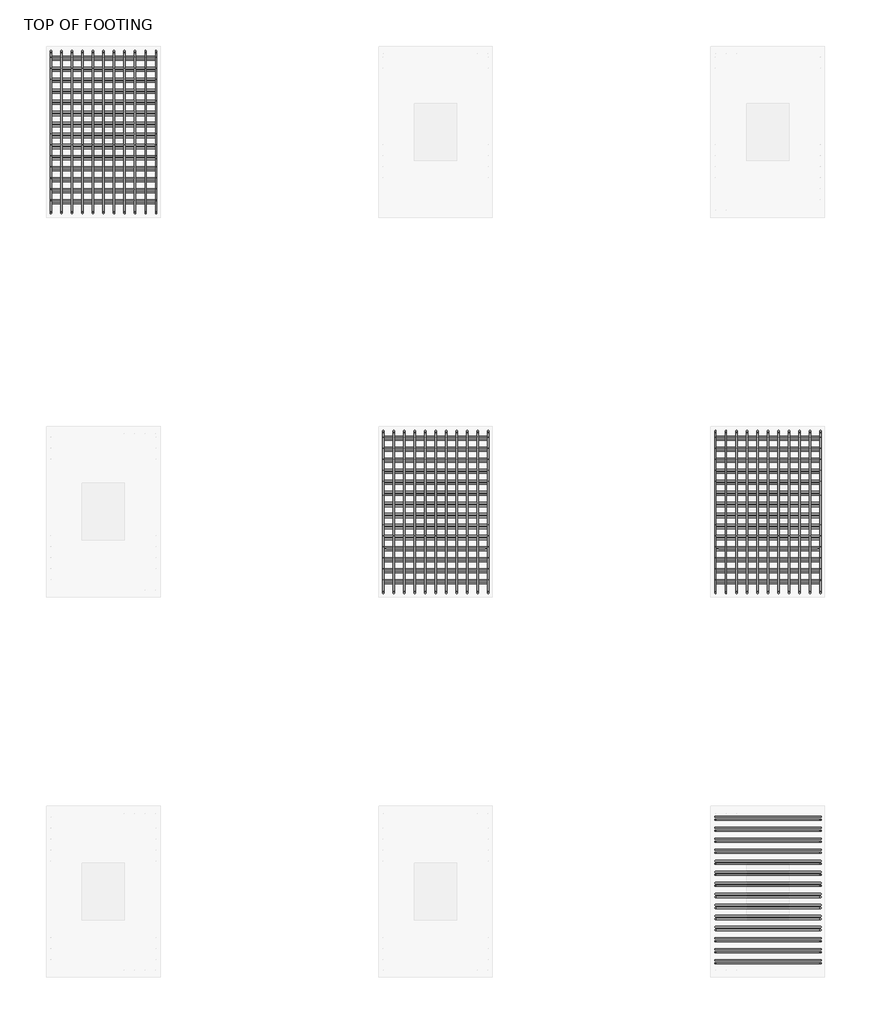
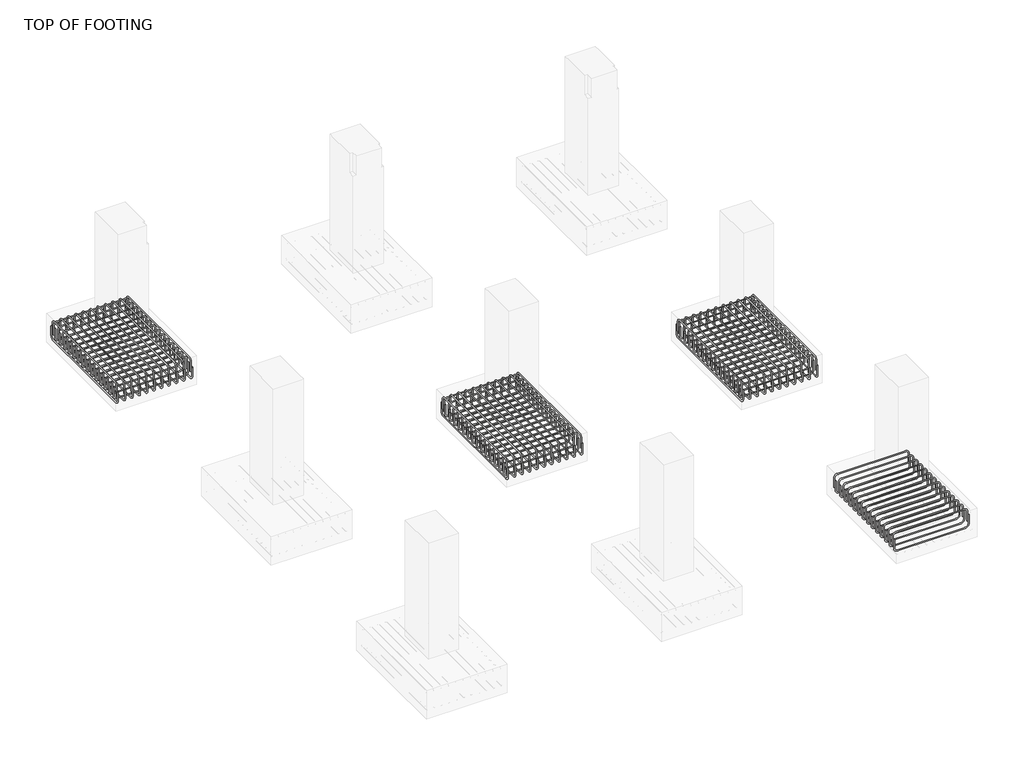
# One storey, part 4 of 11: 14 reinforcing bars.
"""IFC4 building model written with IfcOpenShell, lengths in millimetres."""

from ifc_helpers import new_model, si_unit, point, frame, origin, place, context, project, spatial, polyline, circle_curve, trimmed, segment, composite_curve, source, transform, mapped, element, save
from ifc_brep_helpers import swept_disk

model = new_model("IFC4")

# Units and contexts
model_context = context("Model", 3, world=origin())
ifc_project = project(units=[si_unit("LENGTHUNIT", "METRE", prefix="MILLI")], contexts=[model_context])

# Site, building, storey
site = spatial("IfcSite", under=ifc_project)
building = spatial("IfcBuilding", under=site)
storey = spatial("IfcBuildingStorey", under=building, Name="TOP OF FOOTING", Elevation=-1828.8)

# Reinforcing bars
placement = place(None, origin())
reinforcing_bar_shape = source(origin(), model_context, "Body", "SolidModel", [
    swept_disk(composite_curve([segment(polyline([(-8816.2384094, 10549.4712443, -2012.1658531), (-8816.2384094, 10549.4712443, -2159.4658531)]), True, "CONTINUOUS"), segment(trimmed(circle_curve(frame((-8816.2384094, 10595.8212443, -2159.4658531), z_axis=(1.0, 0.0, 0.0), x_axis=(0.0, -46.349999999998545, 0.0)), 46.35), [point((-8816.2384094, 10549.4712443, -2159.4658531))], [point((-8816.2384094, 10595.8212443, -2205.8158531))], True, "CARTESIAN"), True, "CONTINUOUS"), segment(polyline([(-8816.2384094, 10595.8212443, -2205.8158531), (-8816.2384094, 12210.4212443, -2205.8158531)]), True, "CONTINUOUS"), segment(trimmed(circle_curve(frame((-8816.2384094, 12210.4212443, -2159.4658531), z_axis=(1.0, 0.0, 0.0), x_axis=(0.0, 0.0, -46.34999999999991)), 46.35), [point((-8816.2384094, 12210.4212443, -2205.8158531))], [point((-8816.2384094, 12256.7712443, -2159.4658531))], True, "CARTESIAN"), True, "CONTINUOUS"), segment(polyline([(-8816.2384094, 12256.7712443, -2159.4658531), (-8816.2384094, 12256.7712443, -2012.1658531)]), True, "CONTINUOUS")], self_intersect=False), 6.35),
])
element("IfcReinforcingBar", 1, at=placement, inside=storey, context=model_context, shape_type="MappedRepresentation", body=[
    mapped(reinforcing_bar_shape, transform((0.0, 0.0, 0.0), x_axis=(1.0, 0.0, 0.0), y_axis=(0.0, 1.0, 0.0), z_axis=(0.0, 0.0, 1.0))),
    mapped(reinforcing_bar_shape, transform((-110.73, 0.0, 0.0), x_axis=(1.0, 0.0, 0.0), y_axis=(0.0, 1.0, 0.0), z_axis=(0.0, 0.0, 1.0))),
    mapped(reinforcing_bar_shape, transform((-221.46, 0.0, 0.0), x_axis=(1.0, 0.0, 0.0), y_axis=(0.0, 1.0, 0.0), z_axis=(0.0, 0.0, 1.0))),
    mapped(reinforcing_bar_shape, transform((-332.19, 0.0, 0.0), x_axis=(1.0, 0.0, 0.0), y_axis=(0.0, 1.0, 0.0), z_axis=(0.0, 0.0, 1.0))),
    mapped(reinforcing_bar_shape, transform((-442.92, 0.0, 0.0), x_axis=(1.0, 0.0, 0.0), y_axis=(0.0, 1.0, 0.0), z_axis=(0.0, 0.0, 1.0))),
    mapped(reinforcing_bar_shape, transform((-553.65, 0.0, 0.0), x_axis=(1.0, 0.0, 0.0), y_axis=(0.0, 1.0, 0.0), z_axis=(0.0, 0.0, 1.0))),
    mapped(reinforcing_bar_shape, transform((-664.38, 0.0, 0.0), x_axis=(1.0, 0.0, 0.0), y_axis=(0.0, 1.0, 0.0), z_axis=(0.0, 0.0, 1.0))),
    mapped(reinforcing_bar_shape, transform((-775.11, 0.0, 0.0), x_axis=(1.0, 0.0, 0.0), y_axis=(0.0, 1.0, 0.0), z_axis=(0.0, 0.0, 1.0))),
    mapped(reinforcing_bar_shape, transform((-885.84, 0.0, 0.0), x_axis=(1.0, 0.0, 0.0), y_axis=(0.0, 1.0, 0.0), z_axis=(0.0, 0.0, 1.0))),
    mapped(reinforcing_bar_shape, transform((-996.57, 0.0, 0.0), x_axis=(1.0, 0.0, 0.0), y_axis=(0.0, 1.0, 0.0), z_axis=(0.0, 0.0, 1.0))),
    mapped(reinforcing_bar_shape, transform((-1107.3, 0.0, 0.0), x_axis=(1.0, 0.0, 0.0), y_axis=(0.0, 1.0, 0.0), z_axis=(0.0, 0.0, 1.0))),
])
reinforcing_bar_2_shape = source(origin(), model_context, "Body", "SolidModel", [
    swept_disk(composite_curve([segment(polyline([(-9923.5384094, 10577.6603603, -2096.8914539), (-9923.5384094, 10577.6603603, -1949.5914539)]), True, "CONTINUOUS"), segment(trimmed(circle_curve(frame((-9923.5384094, 10624.0103603, -1949.5914539), z_axis=(-1.0, 0.0, 0.0), x_axis=(0.0, -46.350000000000364, 0.0)), 46.35), [point((-9923.5384094, 10577.6603603, -1949.5914539))], [point((-9923.5384094, 10624.0103603, -1903.2414539))], True, "CARTESIAN"), True, "CONTINUOUS"), segment(polyline([(-9923.5384094, 10624.0103603, -1903.2414539), (-9923.5384094, 12181.3238837, -1903.2414539)]), True, "CONTINUOUS"), segment(trimmed(circle_curve(frame((-9923.5384094, 12181.3238837, -1949.5914539), z_axis=(-1.0, 0.0, 0.0), x_axis=(0.0, 0.0, 46.350000000000136)), 46.35), [point((-9923.5384094, 12181.3238837, -1903.2414539))], [point((-9923.5384094, 12227.6738837, -1949.5914539))], True, "CARTESIAN"), True, "CONTINUOUS"), segment(polyline([(-9923.5384094, 12227.6738837, -1949.5914539), (-9923.5384094, 12227.6738837, -2096.8914539)]), True, "CONTINUOUS")], self_intersect=False), 6.35),
])
element("IfcReinforcingBar", 2, at=placement, inside=storey, context=model_context, shape_type="MappedRepresentation", body=[
    mapped(reinforcing_bar_2_shape, transform((0.0, 0.0, 0.0), x_axis=(1.0, 0.0, 0.0), y_axis=(0.0, 1.0, 0.0), z_axis=(0.0, 0.0, 1.0))),
    mapped(reinforcing_bar_2_shape, transform((110.73, 0.0, 0.0), x_axis=(1.0, 0.0, 0.0), y_axis=(0.0, 1.0, 0.0), z_axis=(0.0, 0.0, 1.0))),
    mapped(reinforcing_bar_2_shape, transform((221.46, 0.0, 0.0), x_axis=(1.0, 0.0, 0.0), y_axis=(0.0, 1.0, 0.0), z_axis=(0.0, 0.0, 1.0))),
    mapped(reinforcing_bar_2_shape, transform((332.19, 0.0, 0.0), x_axis=(1.0, 0.0, 0.0), y_axis=(0.0, 1.0, 0.0), z_axis=(0.0, 0.0, 1.0))),
    mapped(reinforcing_bar_2_shape, transform((442.92, 0.0, 0.0), x_axis=(1.0, 0.0, 0.0), y_axis=(0.0, 1.0, 0.0), z_axis=(0.0, 0.0, 1.0))),
    mapped(reinforcing_bar_2_shape, transform((553.65, 0.0, 0.0), x_axis=(1.0, 0.0, 0.0), y_axis=(0.0, 1.0, 0.0), z_axis=(0.0, 0.0, 1.0))),
    mapped(reinforcing_bar_2_shape, transform((664.38, 0.0, 0.0), x_axis=(1.0, 0.0, 0.0), y_axis=(0.0, 1.0, 0.0), z_axis=(0.0, 0.0, 1.0))),
    mapped(reinforcing_bar_2_shape, transform((775.11, 0.0, 0.0), x_axis=(1.0, 0.0, 0.0), y_axis=(0.0, 1.0, 0.0), z_axis=(0.0, 0.0, 1.0))),
    mapped(reinforcing_bar_2_shape, transform((885.84, 0.0, 0.0), x_axis=(1.0, 0.0, 0.0), y_axis=(0.0, 1.0, 0.0), z_axis=(0.0, 0.0, 1.0))),
    mapped(reinforcing_bar_2_shape, transform((996.57, 0.0, 0.0), x_axis=(1.0, 0.0, 0.0), y_axis=(0.0, 1.0, 0.0), z_axis=(0.0, 0.0, 1.0))),
    mapped(reinforcing_bar_2_shape, transform((1107.3, 0.0, 0.0), x_axis=(1.0, 0.0, 0.0), y_axis=(0.0, 1.0, 0.0), z_axis=(0.0, 0.0, 1.0))),
])
reinforcing_bar_3_shape = source(origin(), model_context, "Body", "SolidModel", [
    swept_disk(composite_curve([segment(polyline([(-9923.5384094, 10653.1930221, -1996.7664426), (-9923.5384094, 10653.1930221, -2144.0664426)]), True, "CONTINUOUS"), segment(trimmed(circle_curve(frame((-9877.1884094, 10653.1930221, -2144.0664426), z_axis=(0.0, -1.0, 0.0), x_axis=(-46.350000000000364, 0.0, 0.0)), 46.35), [point((-9923.5384094, 10653.1930221, -2144.0664426))], [point((-9877.1884094, 10653.1930221, -2190.4164426))], True, "CARTESIAN"), True, "CONTINUOUS"), segment(polyline([(-9877.1884094, 10653.1930221, -2190.4164426), (-8862.5884094, 10653.1930221, -2190.4164426)]), True, "CONTINUOUS"), segment(trimmed(circle_curve(frame((-8862.5884094, 10653.1930221, -2144.0664426), z_axis=(0.0, -1.0, 0.0), x_axis=(0.0, 0.0, -46.350000000000364)), 46.35), [point((-8862.5884094, 10653.1930221, -2190.4164426))], [point((-8816.2384094, 10653.1930221, -2144.0664426))], True, "CARTESIAN"), True, "CONTINUOUS"), segment(polyline([(-8816.2384094, 10653.1930221, -2144.0664426), (-8816.2384094, 10653.1930221, -1996.7664426)]), True, "CONTINUOUS")], self_intersect=False), 6.35),
])
element("IfcReinforcingBar", 3, at=placement, inside=storey, context=model_context, shape_type="MappedRepresentation", body=[
    mapped(reinforcing_bar_3_shape, transform((0.0, 0.0, 0.0), x_axis=(1.0, 0.0, 0.0), y_axis=(0.0, 1.0, 0.0), z_axis=(0.0, 0.0, 1.0))),
    mapped(reinforcing_bar_3_shape, transform((0.0, 116.2744005, 0.0), x_axis=(1.0, 0.0, 0.0), y_axis=(0.0, 1.0, 0.0), z_axis=(0.0, 0.0, 1.0))),
    mapped(reinforcing_bar_3_shape, transform((0.0, 232.5488009, 0.0), x_axis=(1.0, 0.0, 0.0), y_axis=(0.0, 1.0, 0.0), z_axis=(0.0, 0.0, 1.0))),
    mapped(reinforcing_bar_3_shape, transform((0.0, 348.8232014, 0.0), x_axis=(1.0, 0.0, 0.0), y_axis=(0.0, 1.0, 0.0), z_axis=(0.0, 0.0, 1.0))),
    mapped(reinforcing_bar_3_shape, transform((0.0, 465.0976018, 0.0), x_axis=(1.0, 0.0, 0.0), y_axis=(0.0, 1.0, 0.0), z_axis=(0.0, 0.0, 1.0))),
    mapped(reinforcing_bar_3_shape, transform((0.0, 581.3720023, 0.0), x_axis=(1.0, 0.0, 0.0), y_axis=(0.0, 1.0, 0.0), z_axis=(0.0, 0.0, 1.0))),
    mapped(reinforcing_bar_3_shape, transform((0.0, 697.6464027, 0.0), x_axis=(1.0, 0.0, 0.0), y_axis=(0.0, 1.0, 0.0), z_axis=(0.0, 0.0, 1.0))),
    mapped(reinforcing_bar_3_shape, transform((0.0, 813.9208032, 0.0), x_axis=(1.0, 0.0, 0.0), y_axis=(0.0, 1.0, 0.0), z_axis=(0.0, 0.0, 1.0))),
    mapped(reinforcing_bar_3_shape, transform((0.0, 930.1952036, 0.0), x_axis=(1.0, 0.0, 0.0), y_axis=(0.0, 1.0, 0.0), z_axis=(0.0, 0.0, 1.0))),
    mapped(reinforcing_bar_3_shape, transform((0.0, 1046.4696041, 0.0), x_axis=(1.0, 0.0, 0.0), y_axis=(0.0, 1.0, 0.0), z_axis=(0.0, 0.0, 1.0))),
    mapped(reinforcing_bar_3_shape, transform((0.0, 1162.7440045, 0.0), x_axis=(1.0, 0.0, 0.0), y_axis=(0.0, 1.0, 0.0), z_axis=(0.0, 0.0, 1.0))),
    mapped(reinforcing_bar_3_shape, transform((0.0, 1279.018405, 0.0), x_axis=(1.0, 0.0, 0.0), y_axis=(0.0, 1.0, 0.0), z_axis=(0.0, 0.0, 1.0))),
    mapped(reinforcing_bar_3_shape, transform((0.0, 1395.2928054, 0.0), x_axis=(1.0, 0.0, 0.0), y_axis=(0.0, 1.0, 0.0), z_axis=(0.0, 0.0, 1.0))),
    mapped(reinforcing_bar_3_shape, transform((0.0, 1511.5672059, 0.0), x_axis=(1.0, 0.0, 0.0), y_axis=(0.0, 1.0, 0.0), z_axis=(0.0, 0.0, 1.0))),
])
reinforcing_bar_4_shape = source(origin(), model_context, "Body", "SolidModel", [
    swept_disk(composite_curve([segment(polyline([(-9923.5384094, 12194.4257435, -2114.1958609), (-9923.5384094, 12194.4257435, -1966.8958609)]), True, "CONTINUOUS"), segment(trimmed(circle_curve(frame((-9877.1884094, 12194.4257435, -1966.8958609), z_axis=(0.0, 1.0, 0.0), x_axis=(-46.350000000000364, 0.0, 0.0)), 46.35), [point((-9923.5384094, 12194.4257435, -1966.8958609))], [point((-9877.1884094, 12194.4257435, -1920.5458609))], True, "CARTESIAN"), True, "CONTINUOUS"), segment(polyline([(-9877.1884094, 12194.4257435, -1920.5458609), (-8862.5884094, 12194.4257435, -1920.5458609)]), True, "CONTINUOUS"), segment(trimmed(circle_curve(frame((-8862.5884094, 12194.4257435, -1966.8958609), z_axis=(0.0, 1.0, 0.0), x_axis=(0.0, 0.0, 46.34999999999991)), 46.35), [point((-8862.5884094, 12194.4257435, -1920.5458609))], [point((-8816.2384094, 12194.4257435, -1966.8958609))], True, "CARTESIAN"), True, "CONTINUOUS"), segment(polyline([(-8816.2384094, 12194.4257435, -1966.8958609), (-8816.2384094, 12194.4257435, -2114.1958609)]), True, "CONTINUOUS")], self_intersect=False), 6.35),
])
element("IfcReinforcingBar", 4, at=placement, inside=storey, context=model_context, shape_type="MappedRepresentation", body=[
    mapped(reinforcing_bar_4_shape, transform((0.0, 0.0, 0.0), x_axis=(1.0, 0.0, 0.0), y_axis=(0.0, 1.0, 0.0), z_axis=(0.0, 0.0, 1.0))),
    mapped(reinforcing_bar_4_shape, transform((0.0, -116.1057918, 0.0), x_axis=(1.0, 0.0, 0.0), y_axis=(0.0, 1.0, 0.0), z_axis=(0.0, 0.0, 1.0))),
    mapped(reinforcing_bar_4_shape, transform((0.0, -232.2115836, 0.0), x_axis=(1.0, 0.0, 0.0), y_axis=(0.0, 1.0, 0.0), z_axis=(0.0, 0.0, 1.0))),
    mapped(reinforcing_bar_4_shape, transform((0.0, -348.3173754, 0.0), x_axis=(1.0, 0.0, 0.0), y_axis=(0.0, 1.0, 0.0), z_axis=(0.0, 0.0, 1.0))),
    mapped(reinforcing_bar_4_shape, transform((0.0, -464.4231672, 0.0), x_axis=(1.0, 0.0, 0.0), y_axis=(0.0, 1.0, 0.0), z_axis=(0.0, 0.0, 1.0))),
    mapped(reinforcing_bar_4_shape, transform((0.0, -580.528959, 0.0), x_axis=(1.0, 0.0, 0.0), y_axis=(0.0, 1.0, 0.0), z_axis=(0.0, 0.0, 1.0))),
    mapped(reinforcing_bar_4_shape, transform((0.0, -696.6347508, 0.0), x_axis=(1.0, 0.0, 0.0), y_axis=(0.0, 1.0, 0.0), z_axis=(0.0, 0.0, 1.0))),
    mapped(reinforcing_bar_4_shape, transform((0.0, -812.7405426, 0.0), x_axis=(1.0, 0.0, 0.0), y_axis=(0.0, 1.0, 0.0), z_axis=(0.0, 0.0, 1.0))),
    mapped(reinforcing_bar_4_shape, transform((0.0, -928.8463344, 0.0), x_axis=(1.0, 0.0, 0.0), y_axis=(0.0, 1.0, 0.0), z_axis=(0.0, 0.0, 1.0))),
    mapped(reinforcing_bar_4_shape, transform((0.0, -1044.9521262, 0.0), x_axis=(1.0, 0.0, 0.0), y_axis=(0.0, 1.0, 0.0), z_axis=(0.0, 0.0, 1.0))),
    mapped(reinforcing_bar_4_shape, transform((0.0, -1161.057918, 0.0), x_axis=(1.0, 0.0, 0.0), y_axis=(0.0, 1.0, 0.0), z_axis=(0.0, 0.0, 1.0))),
    mapped(reinforcing_bar_4_shape, transform((0.0, -1277.1637098, 0.0), x_axis=(1.0, 0.0, 0.0), y_axis=(0.0, 1.0, 0.0), z_axis=(0.0, 0.0, 1.0))),
    mapped(reinforcing_bar_4_shape, transform((0.0, -1393.2695016, 0.0), x_axis=(1.0, 0.0, 0.0), y_axis=(0.0, 1.0, 0.0), z_axis=(0.0, 0.0, 1.0))),
    mapped(reinforcing_bar_4_shape, transform((0.0, -1509.3752934, 0.0), x_axis=(1.0, 0.0, 0.0), y_axis=(0.0, 1.0, 0.0), z_axis=(0.0, 0.0, 1.0))),
])
reinforcing_bar_5_shape = source(origin(), model_context, "Body", "SolidModel", [
    swept_disk(composite_curve([segment(polyline([(-5316.2384094, 6549.4712443, -2012.1658531), (-5316.2384094, 6549.4712443, -2159.4658531)]), True, "CONTINUOUS"), segment(trimmed(circle_curve(frame((-5316.2384094, 6595.8212443, -2159.4658531), z_axis=(1.0, 0.0, 0.0), x_axis=(0.0, -46.350000000000364, 0.0)), 46.35), [point((-5316.2384094, 6549.4712443, -2159.4658531))], [point((-5316.2384094, 6595.8212443, -2205.8158531))], True, "CARTESIAN"), True, "CONTINUOUS"), segment(polyline([(-5316.2384094, 6595.8212443, -2205.8158531), (-5316.2384094, 8210.4212443, -2205.8158531)]), True, "CONTINUOUS"), segment(trimmed(circle_curve(frame((-5316.2384094, 8210.4212443, -2159.4658531), z_axis=(1.0, 0.0, 0.0), x_axis=(0.0, 0.0, -46.34999999999991)), 46.35), [point((-5316.2384094, 8210.4212443, -2205.8158531))], [point((-5316.2384094, 8256.7712443, -2159.4658531))], True, "CARTESIAN"), True, "CONTINUOUS"), segment(polyline([(-5316.2384094, 8256.7712443, -2159.4658531), (-5316.2384094, 8256.7712443, -2012.1658531)]), True, "CONTINUOUS")], self_intersect=False), 6.35),
])
element("IfcReinforcingBar", 5, at=placement, inside=storey, context=model_context, shape_type="MappedRepresentation", body=[
    mapped(reinforcing_bar_5_shape, transform((0.0, 0.0, 0.0), x_axis=(1.0, 0.0, 0.0), y_axis=(0.0, 1.0, 0.0), z_axis=(0.0, 0.0, 1.0))),
    mapped(reinforcing_bar_5_shape, transform((-110.73, 0.0, 0.0), x_axis=(1.0, 0.0, 0.0), y_axis=(0.0, 1.0, 0.0), z_axis=(0.0, 0.0, 1.0))),
    mapped(reinforcing_bar_5_shape, transform((-221.46, 0.0, 0.0), x_axis=(1.0, 0.0, 0.0), y_axis=(0.0, 1.0, 0.0), z_axis=(0.0, 0.0, 1.0))),
    mapped(reinforcing_bar_5_shape, transform((-332.19, 0.0, 0.0), x_axis=(1.0, 0.0, 0.0), y_axis=(0.0, 1.0, 0.0), z_axis=(0.0, 0.0, 1.0))),
    mapped(reinforcing_bar_5_shape, transform((-442.92, 0.0, 0.0), x_axis=(1.0, 0.0, 0.0), y_axis=(0.0, 1.0, 0.0), z_axis=(0.0, 0.0, 1.0))),
    mapped(reinforcing_bar_5_shape, transform((-553.65, 0.0, 0.0), x_axis=(1.0, 0.0, 0.0), y_axis=(0.0, 1.0, 0.0), z_axis=(0.0, 0.0, 1.0))),
    mapped(reinforcing_bar_5_shape, transform((-664.38, 0.0, 0.0), x_axis=(1.0, 0.0, 0.0), y_axis=(0.0, 1.0, 0.0), z_axis=(0.0, 0.0, 1.0))),
    mapped(reinforcing_bar_5_shape, transform((-775.11, 0.0, 0.0), x_axis=(1.0, 0.0, 0.0), y_axis=(0.0, 1.0, 0.0), z_axis=(0.0, 0.0, 1.0))),
    mapped(reinforcing_bar_5_shape, transform((-885.84, 0.0, 0.0), x_axis=(1.0, 0.0, 0.0), y_axis=(0.0, 1.0, 0.0), z_axis=(0.0, 0.0, 1.0))),
    mapped(reinforcing_bar_5_shape, transform((-996.57, 0.0, 0.0), x_axis=(1.0, 0.0, 0.0), y_axis=(0.0, 1.0, 0.0), z_axis=(0.0, 0.0, 1.0))),
    mapped(reinforcing_bar_5_shape, transform((-1107.3, 0.0, 0.0), x_axis=(1.0, 0.0, 0.0), y_axis=(0.0, 1.0, 0.0), z_axis=(0.0, 0.0, 1.0))),
])
reinforcing_bar_6_shape = source(origin(), model_context, "Body", "SolidModel", [
    swept_disk(composite_curve([segment(polyline([(-6423.5384094, 6577.6603603, -2096.8914539), (-6423.5384094, 6577.6603603, -1949.5914539)]), True, "CONTINUOUS"), segment(trimmed(circle_curve(frame((-6423.5384094, 6624.0103603, -1949.5914539), z_axis=(-1.0, 0.0, 0.0), x_axis=(0.0, -46.349999999999454, 0.0)), 46.35), [point((-6423.5384094, 6577.6603603, -1949.5914539))], [point((-6423.5384094, 6624.0103603, -1903.2414539))], True, "CARTESIAN"), True, "CONTINUOUS"), segment(polyline([(-6423.5384094, 6624.0103603, -1903.2414539), (-6423.5384094, 8181.3238837, -1903.2414539)]), True, "CONTINUOUS"), segment(trimmed(circle_curve(frame((-6423.5384094, 8181.3238837, -1949.5914539), z_axis=(-1.0, 0.0, 0.0), x_axis=(0.0, 0.0, 46.350000000000136)), 46.35), [point((-6423.5384094, 8181.3238837, -1903.2414539))], [point((-6423.5384094, 8227.6738837, -1949.5914539))], True, "CARTESIAN"), True, "CONTINUOUS"), segment(polyline([(-6423.5384094, 8227.6738837, -1949.5914539), (-6423.5384094, 8227.6738837, -2096.8914539)]), True, "CONTINUOUS")], self_intersect=False), 6.35),
])
element("IfcReinforcingBar", 6, at=placement, inside=storey, context=model_context, shape_type="MappedRepresentation", body=[
    mapped(reinforcing_bar_6_shape, transform((0.0, 0.0, 0.0), x_axis=(1.0, 0.0, 0.0), y_axis=(0.0, 1.0, 0.0), z_axis=(0.0, 0.0, 1.0))),
    mapped(reinforcing_bar_6_shape, transform((110.73, 0.0, 0.0), x_axis=(1.0, 0.0, 0.0), y_axis=(0.0, 1.0, 0.0), z_axis=(0.0, 0.0, 1.0))),
    mapped(reinforcing_bar_6_shape, transform((221.46, 0.0, 0.0), x_axis=(1.0, 0.0, 0.0), y_axis=(0.0, 1.0, 0.0), z_axis=(0.0, 0.0, 1.0))),
    mapped(reinforcing_bar_6_shape, transform((332.19, 0.0, 0.0), x_axis=(1.0, 0.0, 0.0), y_axis=(0.0, 1.0, 0.0), z_axis=(0.0, 0.0, 1.0))),
    mapped(reinforcing_bar_6_shape, transform((442.92, 0.0, 0.0), x_axis=(1.0, 0.0, 0.0), y_axis=(0.0, 1.0, 0.0), z_axis=(0.0, 0.0, 1.0))),
    mapped(reinforcing_bar_6_shape, transform((553.65, 0.0, 0.0), x_axis=(1.0, 0.0, 0.0), y_axis=(0.0, 1.0, 0.0), z_axis=(0.0, 0.0, 1.0))),
    mapped(reinforcing_bar_6_shape, transform((664.38, 0.0, 0.0), x_axis=(1.0, 0.0, 0.0), y_axis=(0.0, 1.0, 0.0), z_axis=(0.0, 0.0, 1.0))),
    mapped(reinforcing_bar_6_shape, transform((775.11, 0.0, 0.0), x_axis=(1.0, 0.0, 0.0), y_axis=(0.0, 1.0, 0.0), z_axis=(0.0, 0.0, 1.0))),
    mapped(reinforcing_bar_6_shape, transform((885.84, 0.0, 0.0), x_axis=(1.0, 0.0, 0.0), y_axis=(0.0, 1.0, 0.0), z_axis=(0.0, 0.0, 1.0))),
    mapped(reinforcing_bar_6_shape, transform((996.57, 0.0, 0.0), x_axis=(1.0, 0.0, 0.0), y_axis=(0.0, 1.0, 0.0), z_axis=(0.0, 0.0, 1.0))),
    mapped(reinforcing_bar_6_shape, transform((1107.3, 0.0, 0.0), x_axis=(1.0, 0.0, 0.0), y_axis=(0.0, 1.0, 0.0), z_axis=(0.0, 0.0, 1.0))),
])
reinforcing_bar_7_shape = source(origin(), model_context, "Body", "SolidModel", [
    swept_disk(composite_curve([segment(polyline([(-6423.5384094, 6653.1930221, -1996.7664426), (-6423.5384094, 6653.1930221, -2144.0664426)]), True, "CONTINUOUS"), segment(trimmed(circle_curve(frame((-6377.1884094, 6653.1930221, -2144.0664426), z_axis=(0.0, -1.0, 0.0), x_axis=(-46.350000000000364, 0.0, 0.0)), 46.35), [point((-6423.5384094, 6653.1930221, -2144.0664426))], [point((-6377.1884094, 6653.1930221, -2190.4164426))], True, "CARTESIAN"), True, "CONTINUOUS"), segment(polyline([(-6377.1884094, 6653.1930221, -2190.4164426), (-5362.5884094, 6653.1930221, -2190.4164426)]), True, "CONTINUOUS"), segment(trimmed(circle_curve(frame((-5362.5884094, 6653.1930221, -2144.0664426), z_axis=(0.0, -1.0, 0.0), x_axis=(0.0, 0.0, -46.350000000000364)), 46.35), [point((-5362.5884094, 6653.1930221, -2190.4164426))], [point((-5316.2384094, 6653.1930221, -2144.0664426))], True, "CARTESIAN"), True, "CONTINUOUS"), segment(polyline([(-5316.2384094, 6653.1930221, -2144.0664426), (-5316.2384094, 6653.1930221, -1996.7664426)]), True, "CONTINUOUS")], self_intersect=False), 6.35),
])
element("IfcReinforcingBar", 7, at=placement, inside=storey, context=model_context, shape_type="MappedRepresentation", body=[
    mapped(reinforcing_bar_7_shape, transform((0.0, 0.0, 0.0), x_axis=(1.0, 0.0, 0.0), y_axis=(0.0, 1.0, 0.0), z_axis=(0.0, 0.0, 1.0))),
    mapped(reinforcing_bar_7_shape, transform((0.0, 116.2744005, 0.0), x_axis=(1.0, 0.0, 0.0), y_axis=(0.0, 1.0, 0.0), z_axis=(0.0, 0.0, 1.0))),
    mapped(reinforcing_bar_7_shape, transform((0.0, 232.5488009, 0.0), x_axis=(1.0, 0.0, 0.0), y_axis=(0.0, 1.0, 0.0), z_axis=(0.0, 0.0, 1.0))),
    mapped(reinforcing_bar_7_shape, transform((0.0, 348.8232014, 0.0), x_axis=(1.0, 0.0, 0.0), y_axis=(0.0, 1.0, 0.0), z_axis=(0.0, 0.0, 1.0))),
    mapped(reinforcing_bar_7_shape, transform((0.0, 465.0976018, 0.0), x_axis=(1.0, 0.0, 0.0), y_axis=(0.0, 1.0, 0.0), z_axis=(0.0, 0.0, 1.0))),
    mapped(reinforcing_bar_7_shape, transform((0.0, 581.3720023, 0.0), x_axis=(1.0, 0.0, 0.0), y_axis=(0.0, 1.0, 0.0), z_axis=(0.0, 0.0, 1.0))),
    mapped(reinforcing_bar_7_shape, transform((0.0, 697.6464027, 0.0), x_axis=(1.0, 0.0, 0.0), y_axis=(0.0, 1.0, 0.0), z_axis=(0.0, 0.0, 1.0))),
    mapped(reinforcing_bar_7_shape, transform((0.0, 813.9208032, 0.0), x_axis=(1.0, 0.0, 0.0), y_axis=(0.0, 1.0, 0.0), z_axis=(0.0, 0.0, 1.0))),
    mapped(reinforcing_bar_7_shape, transform((0.0, 930.1952036, 0.0), x_axis=(1.0, 0.0, 0.0), y_axis=(0.0, 1.0, 0.0), z_axis=(0.0, 0.0, 1.0))),
    mapped(reinforcing_bar_7_shape, transform((0.0, 1046.4696041, 0.0), x_axis=(1.0, 0.0, 0.0), y_axis=(0.0, 1.0, 0.0), z_axis=(0.0, 0.0, 1.0))),
    mapped(reinforcing_bar_7_shape, transform((0.0, 1162.7440045, 0.0), x_axis=(1.0, 0.0, 0.0), y_axis=(0.0, 1.0, 0.0), z_axis=(0.0, 0.0, 1.0))),
    mapped(reinforcing_bar_7_shape, transform((0.0, 1279.018405, 0.0), x_axis=(1.0, 0.0, 0.0), y_axis=(0.0, 1.0, 0.0), z_axis=(0.0, 0.0, 1.0))),
    mapped(reinforcing_bar_7_shape, transform((0.0, 1395.2928054, 0.0), x_axis=(1.0, 0.0, 0.0), y_axis=(0.0, 1.0, 0.0), z_axis=(0.0, 0.0, 1.0))),
    mapped(reinforcing_bar_7_shape, transform((0.0, 1511.5672059, 0.0), x_axis=(1.0, 0.0, 0.0), y_axis=(0.0, 1.0, 0.0), z_axis=(0.0, 0.0, 1.0))),
])
reinforcing_bar_8_shape = source(origin(), model_context, "Body", "SolidModel", [
    swept_disk(composite_curve([segment(polyline([(-6423.5384094, 8194.4257435, -2114.1958609), (-6423.5384094, 8194.4257435, -1966.8958609)]), True, "CONTINUOUS"), segment(trimmed(circle_curve(frame((-6377.1884094, 8194.4257435, -1966.8958609), z_axis=(0.0, 1.0, 0.0), x_axis=(-46.350000000000364, 0.0, 0.0)), 46.35), [point((-6423.5384094, 8194.4257435, -1966.8958609))], [point((-6377.1884094, 8194.4257435, -1920.5458609))], True, "CARTESIAN"), True, "CONTINUOUS"), segment(polyline([(-6377.1884094, 8194.4257435, -1920.5458609), (-5362.5884094, 8194.4257435, -1920.5458609)]), True, "CONTINUOUS"), segment(trimmed(circle_curve(frame((-5362.5884094, 8194.4257435, -1966.8958609), z_axis=(0.0, 1.0, 0.0), x_axis=(0.0, 0.0, 46.34999999999991)), 46.35), [point((-5362.5884094, 8194.4257435, -1920.5458609))], [point((-5316.2384094, 8194.4257435, -1966.8958609))], True, "CARTESIAN"), True, "CONTINUOUS"), segment(polyline([(-5316.2384094, 8194.4257435, -1966.8958609), (-5316.2384094, 8194.4257435, -2114.1958609)]), True, "CONTINUOUS")], self_intersect=False), 6.35),
])
element("IfcReinforcingBar", 8, at=placement, inside=storey, context=model_context, shape_type="MappedRepresentation", body=[
    mapped(reinforcing_bar_8_shape, transform((0.0, 0.0, 0.0), x_axis=(1.0, 0.0, 0.0), y_axis=(0.0, 1.0, 0.0), z_axis=(0.0, 0.0, 1.0))),
    mapped(reinforcing_bar_8_shape, transform((0.0, -116.1057918, 0.0), x_axis=(1.0, 0.0, 0.0), y_axis=(0.0, 1.0, 0.0), z_axis=(0.0, 0.0, 1.0))),
    mapped(reinforcing_bar_8_shape, transform((0.0, -232.2115836, 0.0), x_axis=(1.0, 0.0, 0.0), y_axis=(0.0, 1.0, 0.0), z_axis=(0.0, 0.0, 1.0))),
    mapped(reinforcing_bar_8_shape, transform((0.0, -348.3173754, 0.0), x_axis=(1.0, 0.0, 0.0), y_axis=(0.0, 1.0, 0.0), z_axis=(0.0, 0.0, 1.0))),
    mapped(reinforcing_bar_8_shape, transform((0.0, -464.4231672, 0.0), x_axis=(1.0, 0.0, 0.0), y_axis=(0.0, 1.0, 0.0), z_axis=(0.0, 0.0, 1.0))),
    mapped(reinforcing_bar_8_shape, transform((0.0, -580.528959, 0.0), x_axis=(1.0, 0.0, 0.0), y_axis=(0.0, 1.0, 0.0), z_axis=(0.0, 0.0, 1.0))),
    mapped(reinforcing_bar_8_shape, transform((0.0, -696.6347508, 0.0), x_axis=(1.0, 0.0, 0.0), y_axis=(0.0, 1.0, 0.0), z_axis=(0.0, 0.0, 1.0))),
    mapped(reinforcing_bar_8_shape, transform((0.0, -812.7405426, 0.0), x_axis=(1.0, 0.0, 0.0), y_axis=(0.0, 1.0, 0.0), z_axis=(0.0, 0.0, 1.0))),
    mapped(reinforcing_bar_8_shape, transform((0.0, -928.8463344, 0.0), x_axis=(1.0, 0.0, 0.0), y_axis=(0.0, 1.0, 0.0), z_axis=(0.0, 0.0, 1.0))),
    mapped(reinforcing_bar_8_shape, transform((0.0, -1044.9521262, 0.0), x_axis=(1.0, 0.0, 0.0), y_axis=(0.0, 1.0, 0.0), z_axis=(0.0, 0.0, 1.0))),
    mapped(reinforcing_bar_8_shape, transform((0.0, -1161.057918, 0.0), x_axis=(1.0, 0.0, 0.0), y_axis=(0.0, 1.0, 0.0), z_axis=(0.0, 0.0, 1.0))),
    mapped(reinforcing_bar_8_shape, transform((0.0, -1277.1637098, 0.0), x_axis=(1.0, 0.0, 0.0), y_axis=(0.0, 1.0, 0.0), z_axis=(0.0, 0.0, 1.0))),
    mapped(reinforcing_bar_8_shape, transform((0.0, -1393.2695016, 0.0), x_axis=(1.0, 0.0, 0.0), y_axis=(0.0, 1.0, 0.0), z_axis=(0.0, 0.0, 1.0))),
    mapped(reinforcing_bar_8_shape, transform((0.0, -1509.3752934, 0.0), x_axis=(1.0, 0.0, 0.0), y_axis=(0.0, 1.0, 0.0), z_axis=(0.0, 0.0, 1.0))),
])
reinforcing_bar_9_shape = source(origin(), model_context, "Body", "SolidModel", [
    swept_disk(composite_curve([segment(polyline([(-1816.2384094, 6549.4712443, -2012.1658531), (-1816.2384094, 6549.4712443, -2159.4658531)]), True, "CONTINUOUS"), segment(trimmed(circle_curve(frame((-1816.2384094, 6595.8212443, -2159.4658531), z_axis=(1.0, 0.0, 0.0), x_axis=(0.0, -46.350000000000364, 0.0)), 46.35), [point((-1816.2384094, 6549.4712443, -2159.4658531))], [point((-1816.2384094, 6595.8212443, -2205.8158531))], True, "CARTESIAN"), True, "CONTINUOUS"), segment(polyline([(-1816.2384094, 6595.8212443, -2205.8158531), (-1816.2384094, 8210.4212443, -2205.8158531)]), True, "CONTINUOUS"), segment(trimmed(circle_curve(frame((-1816.2384094, 8210.4212443, -2159.4658531), z_axis=(1.0, 0.0, 0.0), x_axis=(0.0, 0.0, -46.34999999999991)), 46.35), [point((-1816.2384094, 8210.4212443, -2205.8158531))], [point((-1816.2384094, 8256.7712443, -2159.4658531))], True, "CARTESIAN"), True, "CONTINUOUS"), segment(polyline([(-1816.2384094, 8256.7712443, -2159.4658531), (-1816.2384094, 8256.7712443, -2012.1658531)]), True, "CONTINUOUS")], self_intersect=False), 6.35),
])
element("IfcReinforcingBar", 9, at=placement, inside=storey, context=model_context, shape_type="MappedRepresentation", body=[
    mapped(reinforcing_bar_9_shape, transform((0.0, 0.0, 0.0), x_axis=(1.0, 0.0, 0.0), y_axis=(0.0, 1.0, 0.0), z_axis=(0.0, 0.0, 1.0))),
    mapped(reinforcing_bar_9_shape, transform((-110.73, 0.0, 0.0), x_axis=(1.0, 0.0, 0.0), y_axis=(0.0, 1.0, 0.0), z_axis=(0.0, 0.0, 1.0))),
    mapped(reinforcing_bar_9_shape, transform((-221.46, 0.0, 0.0), x_axis=(1.0, 0.0, 0.0), y_axis=(0.0, 1.0, 0.0), z_axis=(0.0, 0.0, 1.0))),
    mapped(reinforcing_bar_9_shape, transform((-332.19, 0.0, 0.0), x_axis=(1.0, 0.0, 0.0), y_axis=(0.0, 1.0, 0.0), z_axis=(0.0, 0.0, 1.0))),
    mapped(reinforcing_bar_9_shape, transform((-442.92, 0.0, 0.0), x_axis=(1.0, 0.0, 0.0), y_axis=(0.0, 1.0, 0.0), z_axis=(0.0, 0.0, 1.0))),
    mapped(reinforcing_bar_9_shape, transform((-553.65, 0.0, 0.0), x_axis=(1.0, 0.0, 0.0), y_axis=(0.0, 1.0, 0.0), z_axis=(0.0, 0.0, 1.0))),
    mapped(reinforcing_bar_9_shape, transform((-664.38, 0.0, 0.0), x_axis=(1.0, 0.0, 0.0), y_axis=(0.0, 1.0, 0.0), z_axis=(0.0, 0.0, 1.0))),
    mapped(reinforcing_bar_9_shape, transform((-775.11, 0.0, 0.0), x_axis=(1.0, 0.0, 0.0), y_axis=(0.0, 1.0, 0.0), z_axis=(0.0, 0.0, 1.0))),
    mapped(reinforcing_bar_9_shape, transform((-885.84, 0.0, 0.0), x_axis=(1.0, 0.0, 0.0), y_axis=(0.0, 1.0, 0.0), z_axis=(0.0, 0.0, 1.0))),
    mapped(reinforcing_bar_9_shape, transform((-996.57, 0.0, 0.0), x_axis=(1.0, 0.0, 0.0), y_axis=(0.0, 1.0, 0.0), z_axis=(0.0, 0.0, 1.0))),
    mapped(reinforcing_bar_9_shape, transform((-1107.3, 0.0, 0.0), x_axis=(1.0, 0.0, 0.0), y_axis=(0.0, 1.0, 0.0), z_axis=(0.0, 0.0, 1.0))),
])
reinforcing_bar_10_shape = source(origin(), model_context, "Body", "SolidModel", [
    swept_disk(composite_curve([segment(polyline([(-2923.5384094, 6577.6603603, -2096.8914539), (-2923.5384094, 6577.6603603, -1949.5914539)]), True, "CONTINUOUS"), segment(trimmed(circle_curve(frame((-2923.5384094, 6624.0103603, -1949.5914539), z_axis=(-1.0, 0.0, 0.0), x_axis=(0.0, -46.349999999999454, 0.0)), 46.35), [point((-2923.5384094, 6577.6603603, -1949.5914539))], [point((-2923.5384094, 6624.0103603, -1903.2414539))], True, "CARTESIAN"), True, "CONTINUOUS"), segment(polyline([(-2923.5384094, 6624.0103603, -1903.2414539), (-2923.5384094, 8181.3238837, -1903.2414539)]), True, "CONTINUOUS"), segment(trimmed(circle_curve(frame((-2923.5384094, 8181.3238837, -1949.5914539), z_axis=(-1.0, 0.0, 0.0), x_axis=(0.0, 0.0, 46.350000000000136)), 46.35), [point((-2923.5384094, 8181.3238837, -1903.2414539))], [point((-2923.5384094, 8227.6738837, -1949.5914539))], True, "CARTESIAN"), True, "CONTINUOUS"), segment(polyline([(-2923.5384094, 8227.6738837, -1949.5914539), (-2923.5384094, 8227.6738837, -2096.8914539)]), True, "CONTINUOUS")], self_intersect=False), 6.35),
])
element("IfcReinforcingBar", 10, at=placement, inside=storey, context=model_context, shape_type="MappedRepresentation", body=[
    mapped(reinforcing_bar_10_shape, transform((0.0, 0.0, 0.0), x_axis=(1.0, 0.0, 0.0), y_axis=(0.0, 1.0, 0.0), z_axis=(0.0, 0.0, 1.0))),
    mapped(reinforcing_bar_10_shape, transform((110.73, 0.0, 0.0), x_axis=(1.0, 0.0, 0.0), y_axis=(0.0, 1.0, 0.0), z_axis=(0.0, 0.0, 1.0))),
    mapped(reinforcing_bar_10_shape, transform((221.46, 0.0, 0.0), x_axis=(1.0, 0.0, 0.0), y_axis=(0.0, 1.0, 0.0), z_axis=(0.0, 0.0, 1.0))),
    mapped(reinforcing_bar_10_shape, transform((332.19, 0.0, 0.0), x_axis=(1.0, 0.0, 0.0), y_axis=(0.0, 1.0, 0.0), z_axis=(0.0, 0.0, 1.0))),
    mapped(reinforcing_bar_10_shape, transform((442.92, 0.0, 0.0), x_axis=(1.0, 0.0, 0.0), y_axis=(0.0, 1.0, 0.0), z_axis=(0.0, 0.0, 1.0))),
    mapped(reinforcing_bar_10_shape, transform((553.65, 0.0, 0.0), x_axis=(1.0, 0.0, 0.0), y_axis=(0.0, 1.0, 0.0), z_axis=(0.0, 0.0, 1.0))),
    mapped(reinforcing_bar_10_shape, transform((664.38, 0.0, 0.0), x_axis=(1.0, 0.0, 0.0), y_axis=(0.0, 1.0, 0.0), z_axis=(0.0, 0.0, 1.0))),
    mapped(reinforcing_bar_10_shape, transform((775.11, 0.0, 0.0), x_axis=(1.0, 0.0, 0.0), y_axis=(0.0, 1.0, 0.0), z_axis=(0.0, 0.0, 1.0))),
    mapped(reinforcing_bar_10_shape, transform((885.84, 0.0, 0.0), x_axis=(1.0, 0.0, 0.0), y_axis=(0.0, 1.0, 0.0), z_axis=(0.0, 0.0, 1.0))),
    mapped(reinforcing_bar_10_shape, transform((996.57, 0.0, 0.0), x_axis=(1.0, 0.0, 0.0), y_axis=(0.0, 1.0, 0.0), z_axis=(0.0, 0.0, 1.0))),
    mapped(reinforcing_bar_10_shape, transform((1107.3, 0.0, 0.0), x_axis=(1.0, 0.0, 0.0), y_axis=(0.0, 1.0, 0.0), z_axis=(0.0, 0.0, 1.0))),
])
reinforcing_bar_11_shape = source(origin(), model_context, "Body", "SolidModel", [
    swept_disk(composite_curve([segment(polyline([(-2923.5384094, 6653.1930221, -1996.7664426), (-2923.5384094, 6653.1930221, -2144.0664426)]), True, "CONTINUOUS"), segment(trimmed(circle_curve(frame((-2877.1884094, 6653.1930221, -2144.0664426), z_axis=(0.0, -1.0, 0.0), x_axis=(-46.34999999999991, 0.0, 0.0)), 46.35), [point((-2923.5384094, 6653.1930221, -2144.0664426))], [point((-2877.1884094, 6653.1930221, -2190.4164426))], True, "CARTESIAN"), True, "CONTINUOUS"), segment(polyline([(-2877.1884094, 6653.1930221, -2190.4164426), (-1862.5884094, 6653.1930221, -2190.4164426)]), True, "CONTINUOUS"), segment(trimmed(circle_curve(frame((-1862.5884094, 6653.1930221, -2144.0664426), z_axis=(0.0, -1.0, 0.0), x_axis=(0.0, 0.0, -46.350000000000364)), 46.35), [point((-1862.5884094, 6653.1930221, -2190.4164426))], [point((-1816.2384094, 6653.1930221, -2144.0664426))], True, "CARTESIAN"), True, "CONTINUOUS"), segment(polyline([(-1816.2384094, 6653.1930221, -2144.0664426), (-1816.2384094, 6653.1930221, -1996.7664426)]), True, "CONTINUOUS")], self_intersect=False), 6.35),
])
element("IfcReinforcingBar", 11, at=placement, inside=storey, context=model_context, shape_type="MappedRepresentation", body=[
    mapped(reinforcing_bar_11_shape, transform((0.0, 0.0, 0.0), x_axis=(1.0, 0.0, 0.0), y_axis=(0.0, 1.0, 0.0), z_axis=(0.0, 0.0, 1.0))),
    mapped(reinforcing_bar_11_shape, transform((0.0, 116.2744005, 0.0), x_axis=(1.0, 0.0, 0.0), y_axis=(0.0, 1.0, 0.0), z_axis=(0.0, 0.0, 1.0))),
    mapped(reinforcing_bar_11_shape, transform((0.0, 232.5488009, 0.0), x_axis=(1.0, 0.0, 0.0), y_axis=(0.0, 1.0, 0.0), z_axis=(0.0, 0.0, 1.0))),
    mapped(reinforcing_bar_11_shape, transform((0.0, 348.8232014, 0.0), x_axis=(1.0, 0.0, 0.0), y_axis=(0.0, 1.0, 0.0), z_axis=(0.0, 0.0, 1.0))),
    mapped(reinforcing_bar_11_shape, transform((0.0, 465.0976018, 0.0), x_axis=(1.0, 0.0, 0.0), y_axis=(0.0, 1.0, 0.0), z_axis=(0.0, 0.0, 1.0))),
    mapped(reinforcing_bar_11_shape, transform((0.0, 581.3720023, 0.0), x_axis=(1.0, 0.0, 0.0), y_axis=(0.0, 1.0, 0.0), z_axis=(0.0, 0.0, 1.0))),
    mapped(reinforcing_bar_11_shape, transform((0.0, 697.6464027, 0.0), x_axis=(1.0, 0.0, 0.0), y_axis=(0.0, 1.0, 0.0), z_axis=(0.0, 0.0, 1.0))),
    mapped(reinforcing_bar_11_shape, transform((0.0, 813.9208032, 0.0), x_axis=(1.0, 0.0, 0.0), y_axis=(0.0, 1.0, 0.0), z_axis=(0.0, 0.0, 1.0))),
    mapped(reinforcing_bar_11_shape, transform((0.0, 930.1952036, 0.0), x_axis=(1.0, 0.0, 0.0), y_axis=(0.0, 1.0, 0.0), z_axis=(0.0, 0.0, 1.0))),
    mapped(reinforcing_bar_11_shape, transform((0.0, 1046.4696041, 0.0), x_axis=(1.0, 0.0, 0.0), y_axis=(0.0, 1.0, 0.0), z_axis=(0.0, 0.0, 1.0))),
    mapped(reinforcing_bar_11_shape, transform((0.0, 1162.7440045, 0.0), x_axis=(1.0, 0.0, 0.0), y_axis=(0.0, 1.0, 0.0), z_axis=(0.0, 0.0, 1.0))),
    mapped(reinforcing_bar_11_shape, transform((0.0, 1279.018405, 0.0), x_axis=(1.0, 0.0, 0.0), y_axis=(0.0, 1.0, 0.0), z_axis=(0.0, 0.0, 1.0))),
    mapped(reinforcing_bar_11_shape, transform((0.0, 1395.2928054, 0.0), x_axis=(1.0, 0.0, 0.0), y_axis=(0.0, 1.0, 0.0), z_axis=(0.0, 0.0, 1.0))),
    mapped(reinforcing_bar_11_shape, transform((0.0, 1511.5672059, 0.0), x_axis=(1.0, 0.0, 0.0), y_axis=(0.0, 1.0, 0.0), z_axis=(0.0, 0.0, 1.0))),
])
reinforcing_bar_12_shape = source(origin(), model_context, "Body", "SolidModel", [
    swept_disk(composite_curve([segment(polyline([(-2923.5384094, 8194.4257435, -2114.1958609), (-2923.5384094, 8194.4257435, -1966.8958609)]), True, "CONTINUOUS"), segment(trimmed(circle_curve(frame((-2877.1884094, 8194.4257435, -1966.8958609), z_axis=(0.0, 1.0, 0.0), x_axis=(-46.34999999999991, 0.0, 0.0)), 46.35), [point((-2923.5384094, 8194.4257435, -1966.8958609))], [point((-2877.1884094, 8194.4257435, -1920.5458609))], True, "CARTESIAN"), True, "CONTINUOUS"), segment(polyline([(-2877.1884094, 8194.4257435, -1920.5458609), (-1862.5884094, 8194.4257435, -1920.5458609)]), True, "CONTINUOUS"), segment(trimmed(circle_curve(frame((-1862.5884094, 8194.4257435, -1966.8958609), z_axis=(0.0, 1.0, 0.0), x_axis=(0.0, 0.0, 46.34999999999991)), 46.35), [point((-1862.5884094, 8194.4257435, -1920.5458609))], [point((-1816.2384094, 8194.4257435, -1966.8958609))], True, "CARTESIAN"), True, "CONTINUOUS"), segment(polyline([(-1816.2384094, 8194.4257435, -1966.8958609), (-1816.2384094, 8194.4257435, -2114.1958609)]), True, "CONTINUOUS")], self_intersect=False), 6.35),
])
element("IfcReinforcingBar", 12, at=placement, inside=storey, context=model_context, shape_type="MappedRepresentation", body=[
    mapped(reinforcing_bar_12_shape, transform((0.0, 0.0, 0.0), x_axis=(1.0, 0.0, 0.0), y_axis=(0.0, 1.0, 0.0), z_axis=(0.0, 0.0, 1.0))),
    mapped(reinforcing_bar_12_shape, transform((0.0, -116.1057918, 0.0), x_axis=(1.0, 0.0, 0.0), y_axis=(0.0, 1.0, 0.0), z_axis=(0.0, 0.0, 1.0))),
    mapped(reinforcing_bar_12_shape, transform((0.0, -232.2115836, 0.0), x_axis=(1.0, 0.0, 0.0), y_axis=(0.0, 1.0, 0.0), z_axis=(0.0, 0.0, 1.0))),
    mapped(reinforcing_bar_12_shape, transform((0.0, -348.3173754, 0.0), x_axis=(1.0, 0.0, 0.0), y_axis=(0.0, 1.0, 0.0), z_axis=(0.0, 0.0, 1.0))),
    mapped(reinforcing_bar_12_shape, transform((0.0, -464.4231672, 0.0), x_axis=(1.0, 0.0, 0.0), y_axis=(0.0, 1.0, 0.0), z_axis=(0.0, 0.0, 1.0))),
    mapped(reinforcing_bar_12_shape, transform((0.0, -580.528959, 0.0), x_axis=(1.0, 0.0, 0.0), y_axis=(0.0, 1.0, 0.0), z_axis=(0.0, 0.0, 1.0))),
    mapped(reinforcing_bar_12_shape, transform((0.0, -696.6347508, 0.0), x_axis=(1.0, 0.0, 0.0), y_axis=(0.0, 1.0, 0.0), z_axis=(0.0, 0.0, 1.0))),
    mapped(reinforcing_bar_12_shape, transform((0.0, -812.7405426, 0.0), x_axis=(1.0, 0.0, 0.0), y_axis=(0.0, 1.0, 0.0), z_axis=(0.0, 0.0, 1.0))),
    mapped(reinforcing_bar_12_shape, transform((0.0, -928.8463344, 0.0), x_axis=(1.0, 0.0, 0.0), y_axis=(0.0, 1.0, 0.0), z_axis=(0.0, 0.0, 1.0))),
    mapped(reinforcing_bar_12_shape, transform((0.0, -1044.9521262, 0.0), x_axis=(1.0, 0.0, 0.0), y_axis=(0.0, 1.0, 0.0), z_axis=(0.0, 0.0, 1.0))),
    mapped(reinforcing_bar_12_shape, transform((0.0, -1161.057918, 0.0), x_axis=(1.0, 0.0, 0.0), y_axis=(0.0, 1.0, 0.0), z_axis=(0.0, 0.0, 1.0))),
    mapped(reinforcing_bar_12_shape, transform((0.0, -1277.1637098, 0.0), x_axis=(1.0, 0.0, 0.0), y_axis=(0.0, 1.0, 0.0), z_axis=(0.0, 0.0, 1.0))),
    mapped(reinforcing_bar_12_shape, transform((0.0, -1393.2695016, 0.0), x_axis=(1.0, 0.0, 0.0), y_axis=(0.0, 1.0, 0.0), z_axis=(0.0, 0.0, 1.0))),
    mapped(reinforcing_bar_12_shape, transform((0.0, -1509.3752934, 0.0), x_axis=(1.0, 0.0, 0.0), y_axis=(0.0, 1.0, 0.0), z_axis=(0.0, 0.0, 1.0))),
])
reinforcing_bar_13_shape = source(origin(), model_context, "Body", "SolidModel", [
    swept_disk(composite_curve([segment(polyline([(-2923.5384094, 2653.1930221, -1996.7664426), (-2923.5384094, 2653.1930221, -2144.0664426)]), True, "CONTINUOUS"), segment(trimmed(circle_curve(frame((-2877.1884094, 2653.1930221, -2144.0664426), z_axis=(0.0, -1.0, 0.0), x_axis=(-46.34999999999991, 0.0, 0.0)), 46.35), [point((-2923.5384094, 2653.1930221, -2144.0664426))], [point((-2877.1884094, 2653.1930221, -2190.4164426))], True, "CARTESIAN"), True, "CONTINUOUS"), segment(polyline([(-2877.1884094, 2653.1930221, -2190.4164426), (-1862.5884094, 2653.1930221, -2190.4164426)]), True, "CONTINUOUS"), segment(trimmed(circle_curve(frame((-1862.5884094, 2653.1930221, -2144.0664426), z_axis=(0.0, -1.0, 0.0), x_axis=(0.0, 0.0, -46.350000000000364)), 46.35), [point((-1862.5884094, 2653.1930221, -2190.4164426))], [point((-1816.2384094, 2653.1930221, -2144.0664426))], True, "CARTESIAN"), True, "CONTINUOUS"), segment(polyline([(-1816.2384094, 2653.1930221, -2144.0664426), (-1816.2384094, 2653.1930221, -1996.7664426)]), True, "CONTINUOUS")], self_intersect=False), 6.35),
])
element("IfcReinforcingBar", 13, at=placement, inside=storey, context=model_context, shape_type="MappedRepresentation", body=[
    mapped(reinforcing_bar_13_shape, transform((0.0, 0.0, 0.0), x_axis=(1.0, 0.0, 0.0), y_axis=(0.0, 1.0, 0.0), z_axis=(0.0, 0.0, 1.0))),
    mapped(reinforcing_bar_13_shape, transform((0.0, 116.2744005, 0.0), x_axis=(1.0, 0.0, 0.0), y_axis=(0.0, 1.0, 0.0), z_axis=(0.0, 0.0, 1.0))),
    mapped(reinforcing_bar_13_shape, transform((0.0, 232.5488009, 0.0), x_axis=(1.0, 0.0, 0.0), y_axis=(0.0, 1.0, 0.0), z_axis=(0.0, 0.0, 1.0))),
    mapped(reinforcing_bar_13_shape, transform((0.0, 348.8232014, 0.0), x_axis=(1.0, 0.0, 0.0), y_axis=(0.0, 1.0, 0.0), z_axis=(0.0, 0.0, 1.0))),
    mapped(reinforcing_bar_13_shape, transform((0.0, 465.0976018, 0.0), x_axis=(1.0, 0.0, 0.0), y_axis=(0.0, 1.0, 0.0), z_axis=(0.0, 0.0, 1.0))),
    mapped(reinforcing_bar_13_shape, transform((0.0, 581.3720023, 0.0), x_axis=(1.0, 0.0, 0.0), y_axis=(0.0, 1.0, 0.0), z_axis=(0.0, 0.0, 1.0))),
    mapped(reinforcing_bar_13_shape, transform((0.0, 697.6464027, 0.0), x_axis=(1.0, 0.0, 0.0), y_axis=(0.0, 1.0, 0.0), z_axis=(0.0, 0.0, 1.0))),
    mapped(reinforcing_bar_13_shape, transform((0.0, 813.9208032, 0.0), x_axis=(1.0, 0.0, 0.0), y_axis=(0.0, 1.0, 0.0), z_axis=(0.0, 0.0, 1.0))),
    mapped(reinforcing_bar_13_shape, transform((0.0, 930.1952036, 0.0), x_axis=(1.0, 0.0, 0.0), y_axis=(0.0, 1.0, 0.0), z_axis=(0.0, 0.0, 1.0))),
    mapped(reinforcing_bar_13_shape, transform((0.0, 1046.4696041, 0.0), x_axis=(1.0, 0.0, 0.0), y_axis=(0.0, 1.0, 0.0), z_axis=(0.0, 0.0, 1.0))),
    mapped(reinforcing_bar_13_shape, transform((0.0, 1162.7440045, 0.0), x_axis=(1.0, 0.0, 0.0), y_axis=(0.0, 1.0, 0.0), z_axis=(0.0, 0.0, 1.0))),
    mapped(reinforcing_bar_13_shape, transform((0.0, 1279.018405, 0.0), x_axis=(1.0, 0.0, 0.0), y_axis=(0.0, 1.0, 0.0), z_axis=(0.0, 0.0, 1.0))),
    mapped(reinforcing_bar_13_shape, transform((0.0, 1395.2928054, 0.0), x_axis=(1.0, 0.0, 0.0), y_axis=(0.0, 1.0, 0.0), z_axis=(0.0, 0.0, 1.0))),
    mapped(reinforcing_bar_13_shape, transform((0.0, 1511.5672059, 0.0), x_axis=(1.0, 0.0, 0.0), y_axis=(0.0, 1.0, 0.0), z_axis=(0.0, 0.0, 1.0))),
])
reinforcing_bar_14_shape = source(origin(), model_context, "Body", "SolidModel", [
    swept_disk(composite_curve([segment(polyline([(-2923.5384094, 4194.4257435, -2114.1958609), (-2923.5384094, 4194.4257435, -1966.8958609)]), True, "CONTINUOUS"), segment(trimmed(circle_curve(frame((-2877.1884094, 4194.4257435, -1966.8958609), z_axis=(0.0, 1.0, 0.0), x_axis=(-46.34999999999991, 0.0, 0.0)), 46.35), [point((-2923.5384094, 4194.4257435, -1966.8958609))], [point((-2877.1884094, 4194.4257435, -1920.5458609))], True, "CARTESIAN"), True, "CONTINUOUS"), segment(polyline([(-2877.1884094, 4194.4257435, -1920.5458609), (-1862.5884094, 4194.4257435, -1920.5458609)]), True, "CONTINUOUS"), segment(trimmed(circle_curve(frame((-1862.5884094, 4194.4257435, -1966.8958609), z_axis=(0.0, 1.0, 0.0), x_axis=(0.0, 0.0, 46.34999999999991)), 46.35), [point((-1862.5884094, 4194.4257435, -1920.5458609))], [point((-1816.2384094, 4194.4257435, -1966.8958609))], True, "CARTESIAN"), True, "CONTINUOUS"), segment(polyline([(-1816.2384094, 4194.4257435, -1966.8958609), (-1816.2384094, 4194.4257435, -2114.1958609)]), True, "CONTINUOUS")], self_intersect=False), 6.35),
])
element("IfcReinforcingBar", 14, at=placement, inside=storey, context=model_context, shape_type="MappedRepresentation", body=[
    mapped(reinforcing_bar_14_shape, transform((0.0, 0.0, 0.0), x_axis=(1.0, 0.0, 0.0), y_axis=(0.0, 1.0, 0.0), z_axis=(0.0, 0.0, 1.0))),
    mapped(reinforcing_bar_14_shape, transform((0.0, -116.1057918, 0.0), x_axis=(1.0, 0.0, 0.0), y_axis=(0.0, 1.0, 0.0), z_axis=(0.0, 0.0, 1.0))),
    mapped(reinforcing_bar_14_shape, transform((0.0, -232.2115836, 0.0), x_axis=(1.0, 0.0, 0.0), y_axis=(0.0, 1.0, 0.0), z_axis=(0.0, 0.0, 1.0))),
    mapped(reinforcing_bar_14_shape, transform((0.0, -348.3173754, 0.0), x_axis=(1.0, 0.0, 0.0), y_axis=(0.0, 1.0, 0.0), z_axis=(0.0, 0.0, 1.0))),
    mapped(reinforcing_bar_14_shape, transform((0.0, -464.4231672, 0.0), x_axis=(1.0, 0.0, 0.0), y_axis=(0.0, 1.0, 0.0), z_axis=(0.0, 0.0, 1.0))),
    mapped(reinforcing_bar_14_shape, transform((0.0, -580.528959, 0.0), x_axis=(1.0, 0.0, 0.0), y_axis=(0.0, 1.0, 0.0), z_axis=(0.0, 0.0, 1.0))),
    mapped(reinforcing_bar_14_shape, transform((0.0, -696.6347508, 0.0), x_axis=(1.0, 0.0, 0.0), y_axis=(0.0, 1.0, 0.0), z_axis=(0.0, 0.0, 1.0))),
    mapped(reinforcing_bar_14_shape, transform((0.0, -812.7405426, 0.0), x_axis=(1.0, 0.0, 0.0), y_axis=(0.0, 1.0, 0.0), z_axis=(0.0, 0.0, 1.0))),
    mapped(reinforcing_bar_14_shape, transform((0.0, -928.8463344, 0.0), x_axis=(1.0, 0.0, 0.0), y_axis=(0.0, 1.0, 0.0), z_axis=(0.0, 0.0, 1.0))),
    mapped(reinforcing_bar_14_shape, transform((0.0, -1044.9521262, 0.0), x_axis=(1.0, 0.0, 0.0), y_axis=(0.0, 1.0, 0.0), z_axis=(0.0, 0.0, 1.0))),
    mapped(reinforcing_bar_14_shape, transform((0.0, -1161.057918, 0.0), x_axis=(1.0, 0.0, 0.0), y_axis=(0.0, 1.0, 0.0), z_axis=(0.0, 0.0, 1.0))),
    mapped(reinforcing_bar_14_shape, transform((0.0, -1277.1637098, 0.0), x_axis=(1.0, 0.0, 0.0), y_axis=(0.0, 1.0, 0.0), z_axis=(0.0, 0.0, 1.0))),
    mapped(reinforcing_bar_14_shape, transform((0.0, -1393.2695016, 0.0), x_axis=(1.0, 0.0, 0.0), y_axis=(0.0, 1.0, 0.0), z_axis=(0.0, 0.0, 1.0))),
    mapped(reinforcing_bar_14_shape, transform((0.0, -1509.3752934, 0.0), x_axis=(1.0, 0.0, 0.0), y_axis=(0.0, 1.0, 0.0), z_axis=(0.0, 0.0, 1.0))),
])

save(model, "model.ifc")

# Revit data of these elements
# Elements 1, 2, 3, 4, 5, 6, 7, 8, 9, 10, 11, 12, 13, 14 (IfcReinforcingBar)
#   Phase Created = New Construction
